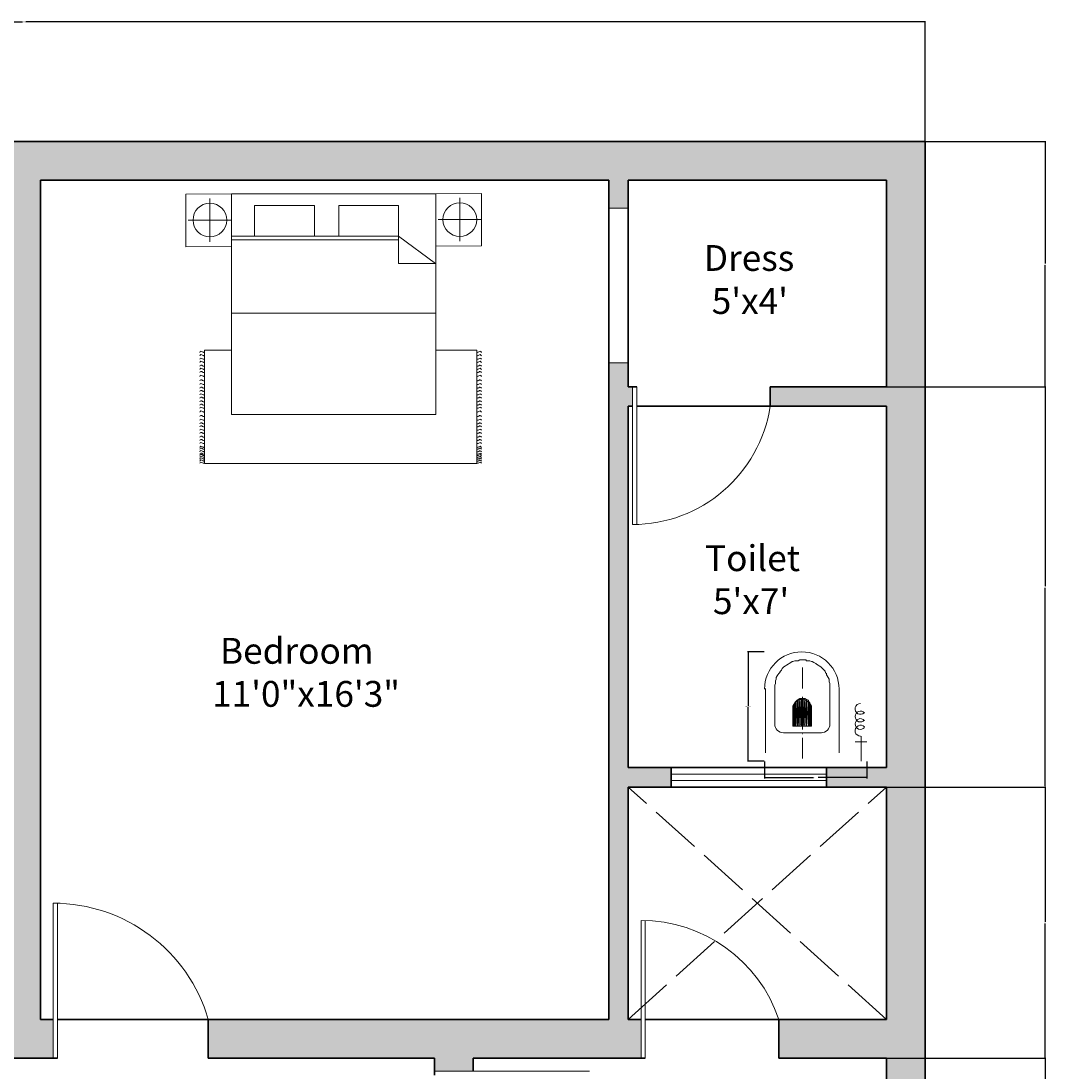
# Model space of a CAD drawing. Units: inches. Extents: x 1752 to 2227, y 6273 to 6884.
# Tile 6 of 6: x 1989 to 2227, y 6640 to 6884. Entities that reach past the tile are written whole.
import ezdxf

# ---------------------------------------------------------------- set-up
doc = ezdxf.new("R2010")
doc.units = ezdxf.units.IN
doc.header["$MEASUREMENT"] = 0
doc.linetypes.add('ACAD_ISO02W100', pattern=[15, 12, -3])
for name, color, linetype, lineweight in [('A-ANNO-DIMS', 2, 'Continuous', 18), ('A-AREA-IDEN', 7, 'Continuous', 18), ('A-DOOR', 3, 'Continuous', 20), ('A-FLOR-FIXT', 8, 'Continuous', 18), ('A-FLOR-VOID', 8, 'ACAD_ISO02W100', 13), ('A-FURN', 8, 'Continuous', 18), ('A-GLAZ', 4, 'Continuous', 18), ('A-WALL', 7, 'Continuous', 35), ('A-WALL-OPNG', 7, 'Continuous', 18)]:
    doc.layers.add(name, color=color, linetype=linetype, lineweight=lineweight)
doc.layers.add('A-WALL-PATT', color=32, linetype='Continuous', lineweight=13, true_color=0xcd6928)
doc.styles.get("Standard").update_dxf_attribs({"font": 'arial.ttf'})
doc.dimstyles.get("Standard").update_dxf_attribs({"dimtxt": 0.18, "dimasz": 0.18, "dimexe": 0.18, "dimexo": 0.0625, "dimgap": 0.09, "dimtad": 0, "dimtih": 1, "dimtoh": 1, "dimdec": 4, "dimzin": 0, "dimdsep": 46, "dimtxsty": 'Standard', "dimcen": 0.09, "dimadec": 0, "dimazin": 0, "dimtfac": 1, "dimtdec": 4, "dimtofl": 0, "dimtmove": 0, "dimatfit": 3, "dimfxl": 1, "dimtolj": 1, "dimtzin": 0, "dimarcsym": 0})

# ---------------------------------------------------------------- blocks, each defined once
blk = doc.blocks.new('BED-DOUBLE-SET')
for p, q in [((5.6, 61.62), (5.6, 51.56)), ((63.65, 61.72), (63.65, 51.66)), ((10.63, 56.59), (0.57, 56.59)), ((68.68, 56.69), (58.62, 56.69)), ((49.39, 52.82), (10.63, 52.82)), ((49.44, 52), (10.63, 52)), ((49.39, 52.82), (58, 46.47)), ((49.44, 52.82), (49.44, 46.47)), ((49.44, 46.47), (58, 46.47)), ((58.05, 34.96), (10.63, 34.96)), ((4.35, 0), (4.35, 26.37)), ((4.35, 26.37), (10.65, 26.37)), ((58.05, 26.37), (67.59, 26.37)), ((67.59, 26.37), (67.59, 0)), ((67.59, 0), (4.35, 0))]:
    blk.add_line(p, q)
for points in [[(0, 50.39), (10.63, 50.5), (10.63, 62.68), (0, 62.58)], [(58.05, 62.68), (58.05, 11.37), (10.63, 11.37), (10.63, 62.68)], [(58.05, 50.5), (68.68, 50.6), (68.68, 62.78), (58.05, 62.68)], [(29.88, 59.98), (29.88, 52.82), (15.98, 52.82), (15.98, 59.98)], [(49.44, 59.98), (49.44, 52.82), (35.55, 52.82), (35.55, 59.98)]]:
    blk.add_lwpolyline(points, close=True)
for centre in [(5.6, 56.59), (63.65, 56.69)]:
    blk.add_circle(centre, 3.92)
for points, knots in [([(3.23, 25.84), (3.32, 25.96), (3.52, 26.2), (3.86, 25.96), (4.14, 25.78), (4.29, 25.89), (4.35, 25.94)], [0, 0, 0, 0, 0.400747, 0.791423, 1.067667, 1.29709, 1.29709, 1.29709, 1.29709]), ([(3.23, 25.06), (3.32, 25.18), (3.52, 25.42), (3.86, 25.18), (4.14, 25.01), (4.29, 25.11), (4.35, 25.16)], [0, 0, 0, 0, 0.400747, 0.791423, 1.067667, 1.29709, 1.29709, 1.29709, 1.29709]), ([(3.23, 24.24), (3.32, 24.36), (3.52, 24.6), (3.86, 24.36), (4.14, 24.19), (4.29, 24.3), (4.35, 24.34)], [0, 0, 0, 0, 0.400747, 0.791423, 1.067667, 1.29709, 1.29709, 1.29709, 1.29709]), ([(68.71, 25.84), (68.61, 25.96), (68.42, 26.2), (68.08, 25.96), (67.8, 25.78), (67.65, 25.89), (67.58, 25.94)], [0, 0, 0, 0, 0.400747, 0.791423, 1.067667, 1.29709, 1.29709, 1.29709, 1.29709]), ([(68.71, 25.06), (68.61, 25.18), (68.42, 25.42), (68.08, 25.18), (67.8, 25.01), (67.65, 25.11), (67.58, 25.16)], [0, 0, 0, 0, 0.400747, 0.791423, 1.067667, 1.29709, 1.29709, 1.29709, 1.29709]), ([(68.71, 24.24), (68.61, 24.36), (68.42, 24.6), (68.08, 24.36), (67.8, 24.19), (67.65, 24.3), (67.58, 24.34)], [0, 0, 0, 0, 0.400747, 0.791423, 1.067667, 1.29709, 1.29709, 1.29709, 1.29709]), ([(3.23, 23.51), (3.32, 23.63), (3.52, 23.87), (3.86, 23.63), (4.14, 23.46), (4.29, 23.57), (4.35, 23.62)], [0, 0, 0, 0, 0.400747, 0.791423, 1.067667, 1.29709, 1.29709, 1.29709, 1.29709]), ([(3.23, 22.63), (3.32, 22.75), (3.52, 22.99), (3.86, 22.75), (4.14, 22.58), (4.29, 22.69), (4.35, 22.73)], [0, 0, 0, 0, 0.400747, 0.791423, 1.067667, 1.29709, 1.29709, 1.29709, 1.29709]), ([(3.23, 21.88), (3.32, 22), (3.52, 22.24), (3.86, 22), (4.14, 21.83), (4.29, 21.93), (4.35, 21.98)], [0, 0, 0, 0, 0.400747, 0.791423, 1.067667, 1.29709, 1.29709, 1.29709, 1.29709]), ([(68.71, 23.51), (68.61, 23.63), (68.42, 23.87), (68.08, 23.63), (67.8, 23.46), (67.65, 23.57), (67.58, 23.62)], [0, 0, 0, 0, 0.400747, 0.791423, 1.067667, 1.29709, 1.29709, 1.29709, 1.29709]), ([(68.71, 22.63), (68.61, 22.75), (68.42, 22.99), (68.08, 22.75), (67.8, 22.58), (67.65, 22.69), (67.58, 22.73)], [0, 0, 0, 0, 0.400747, 0.791423, 1.067667, 1.29709, 1.29709, 1.29709, 1.29709]), ([(68.71, 21.88), (68.61, 22), (68.42, 22.24), (68.08, 22), (67.8, 21.83), (67.65, 21.93), (67.58, 21.98)], [0, 0, 0, 0, 0.400747, 0.791423, 1.067667, 1.29709, 1.29709, 1.29709, 1.29709]), ([(3.23, 21.15), (3.32, 21.27), (3.52, 21.51), (3.86, 21.27), (4.14, 21.1), (4.29, 21.21), (4.35, 21.25)], [0, 0, 0, 0, 0.400747, 0.791423, 1.067667, 1.29709, 1.29709, 1.29709, 1.29709]), ([(3.23, 20.27), (3.32, 20.39), (3.52, 20.63), (3.86, 20.39), (4.14, 20.22), (4.29, 20.32), (4.35, 20.37)], [0, 0, 0, 0, 0.400747, 0.791423, 1.067667, 1.29709, 1.29709, 1.29709, 1.29709]), ([(68.71, 21.15), (68.61, 21.27), (68.42, 21.51), (68.08, 21.27), (67.8, 21.1), (67.65, 21.21), (67.58, 21.25)], [0, 0, 0, 0, 0.400747, 0.791423, 1.067667, 1.29709, 1.29709, 1.29709, 1.29709]), ([(68.71, 20.27), (68.61, 20.39), (68.42, 20.63), (68.08, 20.39), (67.8, 20.22), (67.65, 20.32), (67.58, 20.37)], [0, 0, 0, 0, 0.400747, 0.791423, 1.067667, 1.29709, 1.29709, 1.29709, 1.29709]), ([(3.23, 19.23), (3.32, 19.35), (3.52, 19.59), (3.86, 19.35), (4.14, 19.18), (4.29, 19.29), (4.35, 19.33)], [0, 0, 0, 0, 0.400747, 0.791423, 1.067667, 1.29709, 1.29709, 1.29709, 1.29709]), ([(3.23, 18.35), (3.32, 18.47), (3.52, 18.71), (3.86, 18.47), (4.14, 18.3), (4.29, 18.4), (4.35, 18.45)], [0, 0, 0, 0, 0.400747, 0.791423, 1.067667, 1.29709, 1.29709, 1.29709, 1.29709]), ([(3.23, 17.53), (3.32, 17.65), (3.52, 17.89), (3.86, 17.65), (4.14, 17.48), (4.29, 17.59), (4.35, 17.64)], [0, 0, 0, 0, 0.400747, 0.791423, 1.067667, 1.29709, 1.29709, 1.29709, 1.29709]), ([(68.71, 19.23), (68.61, 19.35), (68.42, 19.59), (68.08, 19.35), (67.8, 19.18), (67.65, 19.29), (67.58, 19.33)], [0, 0, 0, 0, 0.400747, 0.791423, 1.067667, 1.29709, 1.29709, 1.29709, 1.29709]), ([(68.71, 18.35), (68.61, 18.47), (68.42, 18.71), (68.08, 18.47), (67.8, 18.3), (67.65, 18.4), (67.58, 18.45)], [0, 0, 0, 0, 0.400747, 0.791423, 1.067667, 1.29709, 1.29709, 1.29709, 1.29709]), ([(68.71, 17.53), (68.61, 17.65), (68.42, 17.89), (68.08, 17.65), (67.8, 17.48), (67.65, 17.59), (67.58, 17.64)], [0, 0, 0, 0, 0.400747, 0.791423, 1.067667, 1.29709, 1.29709, 1.29709, 1.29709]), ([(3.23, 16.76), (3.32, 16.88), (3.52, 17.12), (3.86, 16.88), (4.14, 16.71), (4.29, 16.81), (4.35, 16.86)], [0, 0, 0, 0, 0.400747, 0.791423, 1.067667, 1.29709, 1.29709, 1.29709, 1.29709]), ([(3.23, 15.94), (3.32, 16.06), (3.52, 16.3), (3.86, 16.06), (4.14, 15.89), (4.29, 16), (4.35, 16.04)], [0, 0, 0, 0, 0.400747, 0.791423, 1.067667, 1.29709, 1.29709, 1.29709, 1.29709]), ([(3.23, 15.21), (3.32, 15.33), (3.52, 15.57), (3.86, 15.33), (4.14, 15.16), (4.29, 15.27), (4.35, 15.32)], [0, 0, 0, 0, 0.400747, 0.791423, 1.067667, 1.29709, 1.29709, 1.29709, 1.29709]), ([(68.71, 16.76), (68.61, 16.88), (68.42, 17.12), (68.08, 16.88), (67.8, 16.71), (67.65, 16.81), (67.58, 16.86)], [0, 0, 0, 0, 0.400747, 0.791423, 1.067667, 1.29709, 1.29709, 1.29709, 1.29709]), ([(68.71, 15.94), (68.61, 16.06), (68.42, 16.3), (68.08, 16.06), (67.8, 15.89), (67.65, 16), (67.58, 16.04)], [0, 0, 0, 0, 0.400747, 0.791423, 1.067667, 1.29709, 1.29709, 1.29709, 1.29709]), ([(68.71, 15.21), (68.61, 15.33), (68.42, 15.57), (68.08, 15.33), (67.8, 15.16), (67.65, 15.27), (67.58, 15.32)], [0, 0, 0, 0, 0.400747, 0.791423, 1.067667, 1.29709, 1.29709, 1.29709, 1.29709]), ([(3.23, 14.33), (3.32, 14.45), (3.52, 14.69), (3.86, 14.45), (4.14, 14.28), (4.29, 14.39), (4.35, 14.43)], [0, 0, 0, 0, 0.400747, 0.791423, 1.067667, 1.29709, 1.29709, 1.29709, 1.29709]), ([(3.23, 13.58), (3.32, 13.7), (3.52, 13.94), (3.86, 13.7), (4.14, 13.53), (4.29, 13.63), (4.35, 13.68)], [0, 0, 0, 0, 0.400747, 0.791423, 1.067667, 1.29709, 1.29709, 1.29709, 1.29709]), ([(3.23, 12.85), (3.32, 12.97), (3.52, 13.21), (3.86, 12.97), (4.14, 12.8), (4.29, 12.9), (4.35, 12.95)], [0, 0, 0, 0, 0.400747, 0.791423, 1.067667, 1.29709, 1.29709, 1.29709, 1.29709]), ([(3.23, 11.97), (3.32, 12.09), (3.52, 12.33), (3.86, 12.09), (4.14, 11.92), (4.29, 12.02), (4.35, 12.07)], [0, 0, 0, 0, 0.400747, 0.791423, 1.067667, 1.29709, 1.29709, 1.29709, 1.29709]), ([(68.71, 14.33), (68.61, 14.45), (68.42, 14.69), (68.08, 14.45), (67.8, 14.28), (67.65, 14.39), (67.58, 14.43)], [0, 0, 0, 0, 0.400747, 0.791423, 1.067667, 1.29709, 1.29709, 1.29709, 1.29709]), ([(68.71, 13.58), (68.61, 13.7), (68.42, 13.94), (68.08, 13.7), (67.8, 13.53), (67.65, 13.63), (67.58, 13.68)], [0, 0, 0, 0, 0.400747, 0.791423, 1.067667, 1.29709, 1.29709, 1.29709, 1.29709]), ([(68.71, 12.85), (68.61, 12.97), (68.42, 13.21), (68.08, 12.97), (67.8, 12.8), (67.65, 12.9), (67.58, 12.95)], [0, 0, 0, 0, 0.400747, 0.791423, 1.067667, 1.29709, 1.29709, 1.29709, 1.29709]), ([(68.71, 11.97), (68.61, 12.09), (68.42, 12.33), (68.08, 12.09), (67.8, 11.92), (67.65, 12.02), (67.58, 12.07)], [0, 0, 0, 0, 0.400747, 0.791423, 1.067667, 1.29709, 1.29709, 1.29709, 1.29709]), ([(3.23, 10.93), (3.32, 11.05), (3.52, 11.29), (3.86, 11.05), (4.14, 10.88), (4.29, 10.99), (4.35, 11.03)], [0, 0, 0, 0, 0.400747, 0.791423, 1.067667, 1.29709, 1.29709, 1.29709, 1.29709]), ([(3.23, 10.05), (3.32, 10.17), (3.52, 10.41), (3.86, 10.17), (4.14, 10), (4.29, 10.1), (4.35, 10.15)], [0, 0, 0, 0, 0.400747, 0.791423, 1.067667, 1.29709, 1.29709, 1.29709, 1.29709]), ([(68.71, 10.93), (68.61, 11.05), (68.42, 11.29), (68.08, 11.05), (67.8, 10.88), (67.65, 10.99), (67.58, 11.03)], [0, 0, 0, 0, 0.400747, 0.791423, 1.067667, 1.29709, 1.29709, 1.29709, 1.29709]), ([(68.71, 10.05), (68.61, 10.17), (68.42, 10.41), (68.08, 10.17), (67.8, 10), (67.65, 10.1), (67.58, 10.15)], [0, 0, 0, 0, 0.400747, 0.791423, 1.067667, 1.29709, 1.29709, 1.29709, 1.29709]), ([(3.23, 9.23), (3.32, 9.35), (3.52, 9.59), (3.86, 9.35), (4.14, 9.18), (4.29, 9.29), (4.35, 9.34)], [0, 0, 0, 0, 0.400747, 0.791423, 1.067667, 1.29709, 1.29709, 1.29709, 1.29709]), ([(3.23, 8.54), (3.32, 8.66), (3.52, 8.9), (3.86, 8.66), (4.14, 8.49), (4.29, 8.6), (4.35, 8.65)], [0, 0, 0, 0, 0.400747, 0.791423, 1.067667, 1.29709, 1.29709, 1.29709, 1.29709]), ([(3.23, 7.73), (3.32, 7.85), (3.52, 8.09), (3.86, 7.85), (4.14, 7.68), (4.29, 7.78), (4.35, 7.83)], [0, 0, 0, 0, 0.400747, 0.791423, 1.067667, 1.29709, 1.29709, 1.29709, 1.29709]), ([(68.71, 9.23), (68.61, 9.35), (68.42, 9.59), (68.08, 9.35), (67.8, 9.18), (67.65, 9.29), (67.58, 9.34)], [0, 0, 0, 0, 0.400747, 0.791423, 1.067667, 1.29709, 1.29709, 1.29709, 1.29709]), ([(68.71, 8.54), (68.61, 8.66), (68.42, 8.9), (68.08, 8.66), (67.8, 8.49), (67.65, 8.6), (67.58, 8.65)], [0, 0, 0, 0, 0.400747, 0.791423, 1.067667, 1.29709, 1.29709, 1.29709, 1.29709]), ([(68.71, 7.73), (68.61, 7.85), (68.42, 8.09), (68.08, 7.85), (67.8, 7.68), (67.65, 7.78), (67.58, 7.83)], [0, 0, 0, 0, 0.400747, 0.791423, 1.067667, 1.29709, 1.29709, 1.29709, 1.29709]), ([(3.23, 7), (3.32, 7.12), (3.52, 7.36), (3.86, 7.12), (4.14, 6.95), (4.29, 7.05), (4.35, 7.1)], [0, 0, 0, 0, 0.400747, 0.791423, 1.067667, 1.29709, 1.29709, 1.29709, 1.29709]), ([(3.23, 6.12), (3.32, 6.24), (3.52, 6.48), (3.86, 6.24), (4.14, 6.07), (4.29, 6.17), (4.35, 6.22)], [0, 0, 0, 0, 0.400747, 0.791423, 1.067667, 1.29709, 1.29709, 1.29709, 1.29709]), ([(3.23, 5.37), (3.32, 5.49), (3.52, 5.73), (3.86, 5.49), (4.14, 5.31), (4.29, 5.42), (4.35, 5.47)], [0, 0, 0, 0, 0.400747, 0.791423, 1.067667, 1.29709, 1.29709, 1.29709, 1.29709]), ([(3.23, 4.64), (3.32, 4.76), (3.52, 5), (3.86, 4.76), (4.14, 4.59), (4.29, 4.69), (4.35, 4.74)], [0, 0, 0, 0, 0.400747, 0.791423, 1.067667, 1.29709, 1.29709, 1.29709, 1.29709]), ([(68.71, 7), (68.61, 7.12), (68.42, 7.36), (68.08, 7.12), (67.8, 6.95), (67.65, 7.05), (67.58, 7.1)], [0, 0, 0, 0, 0.400747, 0.791423, 1.067667, 1.29709, 1.29709, 1.29709, 1.29709]), ([(68.71, 6.12), (68.61, 6.24), (68.42, 6.48), (68.08, 6.24), (67.8, 6.07), (67.65, 6.17), (67.58, 6.22)], [0, 0, 0, 0, 0.400747, 0.791423, 1.067667, 1.29709, 1.29709, 1.29709, 1.29709]), ([(68.71, 5.37), (68.61, 5.49), (68.42, 5.73), (68.08, 5.49), (67.8, 5.31), (67.65, 5.42), (67.58, 5.47)], [0, 0, 0, 0, 0.400747, 0.791423, 1.067667, 1.29709, 1.29709, 1.29709, 1.29709]), ([(68.71, 4.64), (68.61, 4.76), (68.42, 5), (68.08, 4.76), (67.8, 4.59), (67.66, 4.69), (67.59, 4.73)], [0, 0, 0, 0, 0.400747, 0.791423, 1.067667, 1.283686, 1.283686, 1.283686, 1.283686]), ([(3.23, 3.75), (3.32, 3.88), (3.52, 4.12), (3.86, 3.88), (4.14, 3.7), (4.29, 3.81), (4.35, 3.86)], [0, 0, 0, 0, 0.400747, 0.791423, 1.067667, 1.29709, 1.29709, 1.29709, 1.29709]), ([(3.23, 3.33), (3.32, 3.45), (3.52, 3.7), (3.86, 3.45), (4.14, 3.27), (4.29, 3.38), (4.35, 3.43)], [0, 0, 0, 0, 0.407265, 0.802015, 1.07826, 1.307683, 1.307683, 1.307683, 1.307683]), ([(3.23, 2.76), (3.32, 2.88), (3.52, 3.12), (3.86, 2.88), (4.14, 2.71), (4.29, 2.81), (4.35, 2.86)], [0, 0, 0, 0, 0.400747, 0.791423, 1.067667, 1.29709, 1.29709, 1.29709, 1.29709]), ([(3.23, 2.19), (3.32, 2.31), (3.52, 2.55), (3.86, 2.31), (4.14, 2.13), (4.29, 2.24), (4.35, 2.29)], [0, 0, 0, 0, 0.400747, 0.791423, 1.067667, 1.29709, 1.29709, 1.29709, 1.29709]), ([(68.71, 3.75), (68.61, 3.88), (68.42, 4.12), (68.08, 3.88), (67.8, 3.7), (67.66, 3.81), (67.59, 3.85)], [0, 0, 0, 0, 0.400747, 0.791423, 1.067667, 1.283686, 1.283686, 1.283686, 1.283686]), ([(68.71, 3.33), (68.61, 3.45), (68.42, 3.69), (68.08, 3.45), (67.8, 3.28), (67.66, 3.38), (67.59, 3.42)], [0, 0, 0, 0, 0.402903, 0.794912, 1.071156, 1.287177, 1.287177, 1.287177, 1.287177]), ([(68.71, 2.73), (68.61, 2.85), (68.42, 3.09), (68.08, 2.85), (67.8, 2.68), (67.66, 2.78), (67.59, 2.83)], [0, 0, 0, 0, 0.400747, 0.791423, 1.067667, 1.283686, 1.283686, 1.283686, 1.283686]), ([(3.23, 1.88), (3.32, 2), (3.52, 2.24), (3.86, 2), (4.14, 1.82), (4.29, 1.93), (4.35, 1.98)], [0, 0, 0, 0, 0.400747, 0.791423, 1.067667, 1.29709, 1.29709, 1.29709, 1.29709]), ([(3.23, 1.46), (3.32, 1.58), (3.52, 1.82), (3.86, 1.58), (4.14, 1.41), (4.29, 1.51), (4.35, 1.56)], [0, 0, 0, 0, 0.400747, 0.791423, 1.067667, 1.29709, 1.29709, 1.29709, 1.29709]), ([(3.23, 1.06), (3.32, 1.18), (3.52, 1.42), (3.86, 1.18), (4.14, 1.01), (4.29, 1.11), (4.35, 1.16)], [0, 0, 0, 0, 0.400747, 0.791423, 1.067667, 1.29709, 1.29709, 1.29709, 1.29709]), ([(3.23, 0.57), (3.32, 0.7), (3.52, 0.94), (3.86, 0.7), (4.14, 0.52), (4.29, 0.63), (4.35, 0.68)], [0, 0, 0, 0, 0.400747, 0.791423, 1.067667, 1.29709, 1.29709, 1.29709, 1.29709]), ([(3.23, 0.07), (3.32, 0.19), (3.52, 0.43), (3.86, 0.19), (4.14, 0.02), (4.29, 0.13), (4.35, 0.18)], [0, 0, 0, 0, 0.400747, 0.791423, 1.067667, 1.29709, 1.29709, 1.29709, 1.29709]), ([(68.71, 1.43), (68.61, 1.55), (68.42, 1.79), (68.08, 1.55), (67.8, 1.38), (67.65, 1.48), (67.58, 1.53)], [0, 0, 0, 0, 0.400747, 0.791423, 1.067667, 1.29709, 1.29709, 1.29709, 1.29709]), ([(68.71, 1.03), (68.61, 1.15), (68.42, 1.39), (68.08, 1.15), (67.8, 0.98), (67.65, 1.09), (67.58, 1.13)], [0, 0, 0, 0, 0.400747, 0.791423, 1.067667, 1.29709, 1.29709, 1.29709, 1.29709]), ([(68.71, 0.55), (68.61, 0.67), (68.42, 0.91), (68.08, 0.67), (67.8, 0.5), (67.65, 0.6), (67.58, 0.65)], [0, 0, 0, 0, 0.400747, 0.791423, 1.067667, 1.29709, 1.29709, 1.29709, 1.29709]), ([(68.71, 0.07), (68.61, 0.19), (68.42, 0.43), (68.08, 0.19), (67.8, 0.02), (67.65, 0.13), (67.58, 0.18)], [0, 0, 0, 0, 0.400747, 0.791423, 1.067667, 1.29709, 1.29709, 1.29709, 1.29709]), ([(68.71, 2.16), (68.61, 2.28), (68.42, 2.52), (68.08, 2.28), (67.8, 2.11), (67.66, 2.21), (67.59, 2.25)], [0, 0, 0, 0, 0.400747, 0.791423, 1.067667, 1.283686, 1.283686, 1.283686, 1.283686]), ([(68.71, 1.85), (68.61, 1.97), (68.42, 2.21), (68.08, 1.97), (67.8, 1.8), (67.66, 1.9), (67.59, 1.94)], [0, 0, 0, 0, 0.400747, 0.791423, 1.067667, 1.283686, 1.283686, 1.283686, 1.283686])]:
    blk.add_open_spline(points, degree=3, knots=knots)
blk = doc.blocks.new('WC-PLAN')
h = blk.add_hatch(color=256)
h.paths.add_polyline_path([(8.12, 16.94), (13.2, 16.94), (8.12, 17.17)])
h.paths.add_polyline_path([(13.2, 16.94), (8.12, 17.17), (12.82, 17.17)])
h.paths.add_polyline_path([(8.12, 17.17), (12.82, 17.17), (12.44, 17.17)])
h = blk.add_hatch(color=256)
h.paths.add_polyline_path([(8.12, 16.71), (13.58, 16.71), (8.12, 16.94)])
h.paths.add_polyline_path([(13.58, 16.71), (8.12, 16.94), (13.2, 16.94)])
h = blk.add_hatch(color=256)
h.paths.add_polyline_path([(8.12, 16.56), (13.81, 16.56), (8.12, 16.71)])
h.paths.add_polyline_path([(13.81, 16.56), (8.12, 16.71), (13.58, 16.71)])
h = blk.add_hatch(color=256)
h.paths.add_polyline_path([(8.12, 16.18), (14.19, 16.18), (8.12, 16.56)])
h.paths.add_polyline_path([(14.19, 16.18), (8.12, 16.56), (13.81, 16.56)])
h = blk.add_hatch(color=256)
h.paths.add_polyline_path([(8.12, 15.95), (14.34, 15.95), (8.12, 16.18)])
h.paths.add_polyline_path([(14.34, 15.95), (8.12, 16.18), (14.19, 16.18)])
h = blk.add_hatch(color=256)
h.paths.add_polyline_path([(8.12, 15.57), (14.56, 15.57), (8.12, 15.95)])
h.paths.add_polyline_path([(14.56, 15.57), (8.12, 15.95), (14.34, 15.95)])
h = blk.add_hatch(color=256)
h.paths.add_polyline_path([(8.12, 15.19), (14.56, 15.19), (8.12, 15.57)])
h.paths.add_polyline_path([(14.56, 15.19), (8.12, 15.57), (14.56, 15.57)])
h = blk.add_hatch(color=256)
h.paths.add_polyline_path([(8.12, 14.81), (14.56, 14.81), (8.12, 15.19)])
h.paths.add_polyline_path([(14.56, 14.81), (8.12, 15.19), (14.56, 15.19)])
h = blk.add_hatch(color=256)
h.paths.add_polyline_path([(8.12, 14.44), (14.56, 14.44), (8.12, 14.81)])
h.paths.add_polyline_path([(14.56, 14.44), (8.12, 14.81), (14.56, 14.81)])
h = blk.add_hatch(color=256)
h.paths.add_polyline_path([(8.12, 14.06), (14.34, 14.06), (8.12, 14.44)])
h.paths.add_polyline_path([(14.34, 14.06), (8.12, 14.44), (14.56, 14.44)])
h = blk.add_hatch(color=256)
h.paths.add_polyline_path([(8.12, 13.6), (14.19, 13.6), (8.12, 14.06)])
h.paths.add_polyline_path([(14.19, 13.6), (8.12, 14.06), (14.34, 14.06)])
h = blk.add_hatch(color=256)
h.paths.add_polyline_path([(8.12, 13.45), (13.81, 13.45), (8.12, 13.6)])
h.paths.add_polyline_path([(13.81, 13.45), (8.12, 13.6), (14.19, 13.6)])
h = blk.add_hatch(color=256)
h.paths.add_polyline_path([(8.12, 13.22), (13.58, 13.22), (8.12, 13.45)])
h.paths.add_polyline_path([(13.58, 13.22), (8.12, 13.45), (13.81, 13.45)])
h = blk.add_hatch(color=256)
h.paths.add_polyline_path([(8.12, 13.07), (13.2, 13.07), (8.12, 13.22)])
h.paths.add_polyline_path([(13.2, 13.07), (8.12, 13.22), (13.58, 13.22)])
h = blk.add_hatch(color=256)
h.paths.add_polyline_path([(8.12, 12.84), (12.82, 12.84), (8.12, 13.07)])
h.paths.add_polyline_path([(12.82, 12.84), (8.12, 13.07), (13.2, 13.07)])
for points in [[(1.9, 23.54), (16.92, 23.54), (16.92, 23.54)], [(8.72, 21.41), (15.93, 21.41), (15.93, 21.41)], [(15.93, 21.41), (16.69, 21.41), (17.3, 21.41), (17.67, 21.41), (18.05, 21.19), (18.43, 21.19), (18.66, 21.19), (19.04, 21.04), (19.42, 21.04), (19.8, 20.81), (20.03, 20.66), (20.41, 20.43), (20.56, 20.28), (20.94, 20.05), (21.16, 19.82), (21.54, 19.67), (21.77, 19.44), (21.92, 19.29), (22.15, 18.91), (22.3, 18.68), (22.53, 18.3), (22.68, 18.08), (22.91, 17.7), (23.14, 17.32), (23.14, 17.17), (23.29, 16.71), (23.29, 16.33), (23.29, 15.95), (23.52, 15.57), (23.52, 14.97), (23.52, 14.21), (23.29, 14.06), (23.29, 13.6), (23.29, 13.22), (23.14, 12.84), (23.14, 12.69), (22.91, 12.31), (22.68, 11.86), (22.53, 11.7), (22.3, 11.33), (22.15, 11.1), (21.92, 10.72), (21.77, 10.57), (21.54, 10.34), (21.16, 9.96), (20.94, 9.73), (20.56, 9.58), (20.41, 9.35), (20.03, 9.35), (19.8, 9.2), (19.42, 8.97), (19.04, 8.75), (18.66, 8.75), (18.43, 8.75), (18.05, 8.59), (17.67, 8.59), (17.3, 8.59), (16.69, 8.59), (15.93, 8.59)], [(6.6, 19.29), (6.6, 10.57), (6.6, 10.57)], [(8.12, 17.17), (8.12, 12.84), (8.12, 12.84)], [(8.12, 17.17), (12.44, 17.17), (12.44, 17.17)], [(0.61, 14.97), (5.46, 14.97), (5.46, 14.97)], [(6.37, 14.97), (6.37, 15.04), (6.37, 15.04)], [(7.36, 14.97), (14.94, 14.97), (14.94, 14.97)], [(8.57, 15.42), (8.5, 15.42), (8.5, 15.42)], [(8.57, 14.97), (8.5, 15.04), (8.5, 15.04)], [(8.57, 15.42), (8.57, 15.19), (8.57, 14.97)], [(8.57, 14.97), (8.57, 14.81), (8.57, 14.59)], [(16.92, 14.97), (21.77, 14.97), (21.77, 14.97)], [(8.12, 12.84), (12.44, 12.84), (12.44, 12.84)], [(8.57, 14.59), (8.5, 14.59), (8.5, 14.59)], [(8.72, 8.59), (15.93, 8.59), (15.93, 8.59)], [(1.9, 6.47), (16.92, 6.47), (16.92, 6.47)], [(4.48, 2.73), (4.48, 0), (4.48, 0)], [(0, 1.37), (5.84, 1.37), (5.84, 1.37)]]:
    blk.add_lwpolyline(points)
for points in [[(8.12, 16.94), (13.2, 16.94), (8.12, 17.17)], [(13.2, 16.94), (8.12, 17.17), (12.82, 17.17)], [(8.12, 17.17), (12.82, 17.17), (12.44, 17.17)], [(12.82, 17.17), (8.12, 17.17), (8.12, 17.17)], [(8.12, 16.71), (13.58, 16.71), (8.12, 16.94)], [(13.58, 16.71), (8.12, 16.94), (13.2, 16.94)], [(8.12, 16.56), (13.81, 16.56), (8.12, 16.71)], [(13.81, 16.56), (8.12, 16.71), (13.58, 16.71)], [(8.12, 16.18), (14.19, 16.18), (8.12, 16.56)], [(14.19, 16.18), (8.12, 16.56), (13.81, 16.56)], [(8.12, 15.95), (14.34, 15.95), (8.12, 16.18)], [(14.34, 15.95), (8.12, 16.18), (14.19, 16.18)], [(8.12, 15.57), (14.56, 15.57), (8.12, 15.95)], [(14.56, 15.57), (8.12, 15.95), (14.34, 15.95)], [(8.12, 15.19), (14.56, 15.19), (8.12, 15.57)], [(14.56, 15.19), (8.12, 15.57), (14.56, 15.57)], [(8.12, 14.81), (14.56, 14.81), (8.12, 15.19)], [(14.56, 14.81), (8.12, 15.19), (14.56, 15.19)], [(8.12, 14.44), (14.56, 14.44), (8.12, 14.81)], [(14.56, 14.44), (8.12, 14.81), (14.56, 14.81)], [(8.12, 14.06), (14.34, 14.06), (8.12, 14.44)], [(14.34, 14.06), (8.12, 14.44), (14.56, 14.44)], [(8.12, 13.6), (14.19, 13.6), (8.12, 14.06)], [(14.19, 13.6), (8.12, 14.06), (14.34, 14.06)], [(8.12, 13.45), (13.81, 13.45), (8.12, 13.6)], [(13.81, 13.45), (8.12, 13.6), (14.19, 13.6)], [(8.12, 13.22), (13.58, 13.22), (8.12, 13.45)], [(13.58, 13.22), (8.12, 13.45), (13.81, 13.45)], [(8.12, 13.07), (13.2, 13.07), (8.12, 13.22)], [(13.2, 13.07), (8.12, 13.22), (13.58, 13.22)], [(8.12, 12.84), (12.82, 12.84), (8.12, 13.07)], [(12.82, 12.84), (8.12, 13.07), (13.2, 13.07)], [(8.12, 12.84), (12.44, 12.84)], [(12.44, 12.84), (8.12, 12.84), (12.82, 12.84)]]:
    blk.add_lwpolyline(points, close=True)
for points, knots in [([(16.76, 6.47), (21.54, 6.47), (25.41, 10.34), (25.41, 15.12), (25.41, 15.12), (25.41, 19.9), (21.54, 23.77), (16.76, 23.77)], [0, 0, 0, 0, 0.125, 0.125, 0.125, 0.125001, 1, 1, 1, 1]), ([(12.29, 13.07), (13.43, 13.07), (14.34, 13.98), (14.34, 15.12), (14.34, 15.12), (14.34, 16.26), (13.43, 17.17), (12.29, 17.17)], [0, 0, 0, 0, 0.125, 0.125, 0.125, 0.125001, 1, 1, 1, 1]), ([(7.97, 0.53), (8.34, 0.91), (8.5, 1.59), (8.19, 2.05), (8.19, 2.05), (7.89, 2.58), (7.36, 2.88), (6.75, 2.73), (6.75, 2.73), (6.22, 2.58), (5.84, 2.05), (5.84, 1.52)], [0, 0, 0, 0, 0.083333, 0.083333, 0.083333, 0.083334, 0.166667, 0.166667, 0.166667, 0.166668, 1, 1, 1, 1]), ([(9.48, 0.61), (9.86, 0.91), (10.01, 1.52), (9.79, 1.97), (9.79, 1.97), (9.63, 2.43), (9.1, 2.73), (8.65, 2.73), (8.65, 2.73), (8.12, 2.73), (7.66, 2.43), (7.43, 1.97), (7.43, 1.97), (7.28, 1.44), (7.43, 0.91), (7.81, 0.53)], [0, 0, 0, 0, 0.0625, 0.0625, 0.0625, 0.062501, 0.125, 0.125, 0.125, 0.125001, 0.1875, 0.1875, 0.1875, 0.187501, 1, 1, 1, 1]), ([(11.23, 0.53), (11.61, 0.91), (11.76, 1.44), (11.53, 1.97), (11.53, 1.97), (11.38, 2.43), (10.92, 2.73), (10.39, 2.73), (10.39, 2.73), (9.86, 2.73), (9.41, 2.43), (9.18, 1.97), (9.18, 1.97), (9.03, 1.44), (9.18, 0.91), (9.56, 0.53)], [0, 0, 0, 0, 0.0625, 0.0625, 0.0625, 0.062501, 0.125, 0.125, 0.125, 0.125001, 0.1875, 0.1875, 0.1875, 0.187501, 1, 1, 1, 1]), ([(13.43, 1.52), (13.43, 2.05), (12.97, 2.58), (12.44, 2.73), (12.44, 2.73), (11.91, 2.88), (11.3, 2.58), (11, 2.12), (11, 2.12), (10.77, 1.59), (10.85, 0.99), (11.23, 0.61)], [0, 0, 0, 0, 0.083333, 0.083333, 0.083333, 0.083334, 0.166667, 0.166667, 0.166667, 0.166668, 1, 1, 1, 1])]:
    blk.add_open_spline(points, degree=3, knots=knots)
for points in [[(8.65, 21.41), (7.51, 21.41), (6.6, 20.5), (6.6, 19.37)], [(6.6, 10.64), (6.6, 9.5), (7.51, 8.59), (8.65, 8.59)]]:
    blk.add_open_spline(points, degree=3)
blk = doc.blocks.new('DOOR-SINGLE-36IN')
for p, q in [((35, 36), (35, 0)), ((36, 0), (36, 36)), ((36, 0), (35, 0))]:
    blk.add_line(p, q)
blk.add_arc((36, -1.5), 37.5, 90, 163.7398)
blk = doc.blocks.new('DOOR-SINGLE-32IN')
for p, q in [((32, 32), (31, 32)), ((31, 0), (31, 32)), ((32, 32), (32, 0))]:
    blk.add_line(p, q)
blk.add_arc((32, 33.76), 33.76, 198.5866, 270)
blk = doc.blocks.new('*D26')
at = {"layer": 'A-ANNO-DIMS', "color": 0, "lineweight": -2, "transparency": 16777216}
for p, q in [((2161.28, 6737.33), (2157.35, 6737.33)), ((2157.53, 6737.15), (2157.53, 6724.81)), ((2157.53, 6712.1), (2157.53, 6724.44)), ((2161.28, 6711.92), (2157.35, 6711.92))]:
    blk.add_line(p, q, dxfattribs=at)
at = {"layer": 'A-ANNO-DIMS', "color": 0, "transparency": 16777216}
for points in [[(2157.5, 6737.15), (2157.56, 6737.15), (2157.53, 6737.33)], [(2157.5, 6712.1), (2157.56, 6712.1), (2157.53, 6711.92)]]:
    blk.add_solid(points, dxfattribs=at)
at = {"layer": 'Defpoints', "color": 0, "transparency": 16777216}
for p in [(2157.53, 6737.33), (2161.34, 6737.33), (2161.34, 6711.92)]:
    blk.add_point(p, dxfattribs=at)
at = {"layer": 'A-ANNO-DIMS', "color": 0, "transparency": 16777216, "insert": (2157.53, 6724.63), "char_height": 0.18, "attachment_point": 5}
blk.add_mtext('\\A1;WC 25 TYP.', dxfattribs=at)
blk = doc.blocks.new('*D27')
at = {"layer": 'A-ANNO-DIMS', "color": 0, "lineweight": -2, "transparency": 16777216}
for p, q in [((2161.34, 6711.86), (2161.34, 6707.93)), ((2185.11, 6711.86), (2185.11, 6707.93)), ((2161.52, 6708.11), (2172.7, 6708.11)), ((2184.93, 6708.11), (2173.76, 6708.11))]:
    blk.add_line(p, q, dxfattribs=at)
at = {"layer": 'A-ANNO-DIMS', "color": 0, "transparency": 16777216}
for points in [[(2161.52, 6708.14), (2161.52, 6708.08), (2161.34, 6708.11)], [(2184.93, 6708.14), (2184.93, 6708.08), (2185.11, 6708.11)]]:
    blk.add_solid(points, dxfattribs=at)
at = {"layer": 'Defpoints', "color": 0, "transparency": 16777216}
for p in [(2161.34, 6711.92), (2185.11, 6711.92), (2161.34, 6708.11)]:
    blk.add_point(p, dxfattribs=at)
at = {"layer": 'A-ANNO-DIMS', "color": 0, "transparency": 16777216, "insert": (2173.23, 6708.11), "char_height": 0.18, "attachment_point": 5}
blk.add_mtext('\\A1;24 TYP.', dxfattribs=at)
blk = doc.blocks.new('*D40')
at = {"layer": 'A-ANNO-DIMS', "color": 0, "lineweight": -2, "transparency": 16777216}
for p, q in [((1780.15, 6855.98), (1780.15, 6883.94)), ((1780.33, 6883.76), (1989, 6883.76)), ((2198.47, 6883.76), (1989.8, 6883.76)), ((2198.65, 6855.98), (2198.65, 6883.94))]:
    blk.add_line(p, q, dxfattribs=at)
at = {"layer": 'A-ANNO-DIMS', "color": 0, "transparency": 16777216}
for points in [[(1780.33, 6883.79), (1780.33, 6883.73), (1780.15, 6883.76)], [(2198.47, 6883.79), (2198.47, 6883.73), (2198.65, 6883.76)]]:
    blk.add_solid(points, dxfattribs=at)
at = {"layer": 'Defpoints', "color": 0, "transparency": 16777216}
for p in [(2198.65, 6883.76), (1780.15, 6855.91), (2198.65, 6855.91)]:
    blk.add_point(p, dxfattribs=at)
at = {"layer": 'A-ANNO-DIMS', "color": 0, "transparency": 16777216, "insert": (1989.4, 6883.76), "char_height": 0.18, "attachment_point": 5}
blk.add_mtext('\\A1;418.5', dxfattribs=at)
blk = doc.blocks.new('*D43')
at = {"layer": 'A-ANNO-DIMS', "color": 0, "lineweight": -2, "transparency": 16777216}
for p, q in [((2189.71, 6642.91), (2226.68, 6642.91)), ((2226.5, 6642.73), (2226.5, 6572.59)), ((2226.5, 6502.09), (2226.5, 6572.23)), ((2189.71, 6501.91), (2226.68, 6501.91))]:
    blk.add_line(p, q, dxfattribs=at)
at = {"layer": 'A-ANNO-DIMS', "color": 0, "transparency": 16777216}
for points in [[(2226.47, 6642.73), (2226.53, 6642.73), (2226.5, 6642.91)], [(2226.47, 6502.09), (2226.53, 6502.09), (2226.5, 6501.91)]]:
    blk.add_solid(points, dxfattribs=at)
at = {"layer": 'Defpoints', "color": 0, "transparency": 16777216}
for p in [(2189.65, 6642.91), (2226.5, 6642.91), (2189.65, 6501.91)]:
    blk.add_point(p, dxfattribs=at)
at = {"layer": 'A-ANNO-DIMS', "color": 0, "transparency": 16777216, "insert": (2226.5, 6572.41), "char_height": 0.18, "attachment_point": 5}
blk.add_mtext('\\A1;141', dxfattribs=at)
blk = doc.blocks.new('*D44')
at = {"layer": 'A-ANNO-DIMS', "color": 0, "lineweight": -2, "transparency": 16777216}
for p, q in [((2189.71, 6705.91), (2226.68, 6705.91)), ((2226.5, 6705.73), (2226.5, 6674.6)), ((2226.5, 6643.09), (2226.5, 6674.23)), ((2189.71, 6642.91), (2226.68, 6642.91))]:
    blk.add_line(p, q, dxfattribs=at)
at = {"layer": 'A-ANNO-DIMS', "color": 0, "transparency": 16777216}
for points in [[(2226.47, 6705.73), (2226.53, 6705.73), (2226.5, 6705.91)], [(2226.47, 6643.09), (2226.53, 6643.09), (2226.5, 6642.91)]]:
    blk.add_solid(points, dxfattribs=at)
at = {"layer": 'Defpoints', "color": 0, "transparency": 16777216}
for p in [(2189.65, 6705.91), (2226.5, 6705.91), (2189.65, 6642.91)]:
    blk.add_point(p, dxfattribs=at)
at = {"layer": 'A-ANNO-DIMS', "color": 0, "transparency": 16777216, "insert": (2226.5, 6674.41), "char_height": 0.18, "attachment_point": 5}
blk.add_mtext('\\A1;63', dxfattribs=at)
blk = doc.blocks.new('*D45')
at = {"layer": 'A-ANNO-DIMS', "color": 0, "lineweight": -2, "transparency": 16777216}
for p, q in [((2189.71, 6798.91), (2226.68, 6798.91)), ((2226.5, 6798.73), (2226.5, 6752.6)), ((2226.5, 6706.09), (2226.5, 6752.23)), ((2189.71, 6705.91), (2226.68, 6705.91))]:
    blk.add_line(p, q, dxfattribs=at)
at = {"layer": 'A-ANNO-DIMS', "color": 0, "transparency": 16777216}
for points in [[(2226.47, 6798.73), (2226.53, 6798.73), (2226.5, 6798.91)], [(2226.47, 6706.09), (2226.53, 6706.09), (2226.5, 6705.91)]]:
    blk.add_solid(points, dxfattribs=at)
at = {"layer": 'Defpoints', "color": 0, "transparency": 16777216}
for p in [(2189.65, 6798.91), (2226.5, 6798.91), (2189.65, 6705.91)]:
    blk.add_point(p, dxfattribs=at)
at = {"layer": 'A-ANNO-DIMS', "color": 0, "transparency": 16777216, "insert": (2226.5, 6752.41), "char_height": 0.18, "attachment_point": 5}
blk.add_mtext('\\A1;93', dxfattribs=at)
blk = doc.blocks.new('*D46')
at = {"layer": 'A-ANNO-DIMS', "color": 0, "lineweight": -2, "transparency": 16777216}
for p, q in [((2198.71, 6855.91), (2226.68, 6855.91)), ((2226.5, 6855.73), (2226.5, 6827.6)), ((2226.5, 6799.09), (2226.5, 6827.23)), ((2189.71, 6798.91), (2226.68, 6798.91))]:
    blk.add_line(p, q, dxfattribs=at)
at = {"layer": 'A-ANNO-DIMS', "color": 0, "transparency": 16777216}
for points in [[(2226.47, 6855.73), (2226.53, 6855.73), (2226.5, 6855.91)], [(2226.47, 6799.09), (2226.53, 6799.09), (2226.5, 6798.91)]]:
    blk.add_solid(points, dxfattribs=at)
at = {"layer": 'Defpoints', "color": 0, "transparency": 16777216}
for p in [(2198.65, 6855.91), (2226.5, 6855.91), (2189.65, 6798.91)]:
    blk.add_point(p, dxfattribs=at)
at = {"layer": 'A-ANNO-DIMS', "color": 0, "transparency": 16777216, "insert": (2226.5, 6827.41), "char_height": 0.18, "attachment_point": 5}
blk.add_mtext('\\A1;57', dxfattribs=at)

msp = doc.modelspace()

# ---------------------------------------------------------------- hatches: boundary and pattern name
at = {"layer": 'A-WALL-PATT'}
h = msp.add_hatch(color=256, dxfattribs=at)
h.dxf.hatch_style = 1
h.paths.add_polyline_path([(2198.6473, 6855.914), (1780.1473, 6855.914), (1780.1473, 6309.914), (1824.3861, 6309.914), (1824.3861, 6318.914), (1789.1473, 6318.914), (1789.1473, 6501.914), (1790.1473, 6501.914), (1790.1473, 6510.914), (1789.1473, 6510.914), (1789.1473, 6570.914), (1838.6473, 6570.914), (1838.6473, 6510.914), (1822.1473, 6510.914), (1822.1473, 6501.914), (1921.1473, 6501.914), (1921.1473, 6498.914), (1930.1473, 6498.914), (1930.1473, 6501.914), (1930.1473, 6510.914), (1847.6473, 6510.914), (1847.6473, 6585.039), (1838.6473, 6585.039), (1838.6473, 6575.414), (1789.1473, 6575.414), (1789.1473, 6705.914), (1795.2039, 6705.914), (1795.2039, 6714.914), (1789.1473, 6714.914), (1789.1473, 6846.914), (1984.1473, 6846.914), (1984.1473, 6714.914), (1977.8419, 6714.914), (1977.8419, 6705.914), (1984.1473, 6705.914), (1984.1473, 6651.914), (1977.6147, 6651.914), (1977.6147, 6642.914), (1996.1473, 6642.914), (1996.1473, 6651.914), (1993.1473, 6651.914), (1993.1473, 6846.914), (2125.1473, 6846.914), (2125.1473, 6840.4779), (2129.6473, 6840.4779), (2129.6473, 6846.914), (2189.6473, 6846.914), (2189.6473, 6798.914), (2162.6473, 6798.914), (2162.6473, 6794.414), (2189.6473, 6794.414), (2189.6473, 6710.414), (2175.6868, 6710.414), (2175.6868, 6705.914), (2189.6473, 6705.914), (2189.6473, 6651.914), (2164.6473, 6651.914), (2164.6473, 6642.914), (2189.6473, 6642.914), (2189.6473, 6510.914), (2166.7624, 6510.914), (2166.7624, 6501.914), (2189.6473, 6501.914), (2189.6473, 6318.914), (2173.9269, 6318.914), (2173.9269, 6309.914), (2198.6473, 6309.914)])
h.paths.add_polyline_path([(2023.6785, 6318.914), (1930.1473, 6318.914), (1930.1473, 6321.914), (1921.1473, 6321.914), (1921.1473, 6318.914), (1872.3861, 6318.914), (1872.3861, 6309.914), (2023.6785, 6309.914)], flags=17)
h.paths.add_polyline_path([(2092.7496, 6318.914), (2061.7431, 6318.914), (2061.7431, 6309.914), (2092.7496, 6309.914)], flags=0)
h.paths.add_polyline_path([(1947.0033, 6375.914), (1930.1473, 6375.914), (1930.1473, 6462.914), (1921.1473, 6462.914), (1921.1473, 6357.914), (1930.1473, 6357.914), (1930.1473, 6366.914), (1947.0033, 6366.914)], flags=17)
h.paths.add_polyline_path([(2024.6473, 6432.914), (2015.6473, 6432.914), (2015.6473, 6375.914), (1995.0033, 6375.914), (1995.0033, 6366.914), (2024.6473, 6366.914)], flags=17)
h.paths.add_polyline_path([(2030.6473, 6441.914), (2024.6473, 6441.914), (2024.6473, 6510.914), (2015.6473, 6510.914), (2015.6473, 6432.914), (2024.6473, 6432.914), (2030.6473, 6432.914)], flags=17)
h.paths.add_polyline_path([(2093.6473, 6501.914), (2118.7624, 6501.914), (2118.7624, 6510.914), (2093.6473, 6510.914), (2093.6473, 6603.914), (2084.6473, 6603.914), (2084.6473, 6441.914), (2078.6473, 6441.914), (2078.6473, 6432.914), (2093.6473, 6432.914)], flags=17)
h.paths.add_polyline_path([(2132.6473, 6651.914), (2129.6473, 6651.914), (2129.6473, 6705.914), (2139.6868, 6705.914), (2139.6868, 6710.414), (2129.6473, 6710.414), (2129.6473, 6794.414), (2130.6473, 6794.414), (2130.6473, 6798.914), (2129.6473, 6798.914), (2129.6473, 6804.4779), (2125.1473, 6804.4779), (2125.1473, 6651.914), (2032.1473, 6651.914), (2032.1473, 6642.914), (2084.6473, 6642.914), (2084.6473, 6639.914), (2093.6473, 6639.914), (2093.6473, 6642.914), (2132.6473, 6642.914)], flags=17)
h.paths.add_polyline_path([(1929.6147, 6651.914), (1924.1473, 6651.914), (1924.1473, 6705.914), (1941.8419, 6705.914), (1941.8419, 6714.914), (1911.8299, 6714.914), (1911.8299, 6705.914), (1919.6473, 6705.914), (1919.6473, 6651.914), (1847.6473, 6651.914), (1847.6473, 6662.4635), (1838.6473, 6662.4635), (1838.6473, 6621.039), (1847.6473, 6621.039), (1847.6473, 6642.914), (1929.6147, 6642.914)], flags=17)
h.paths.add_polyline_path([(1879.8299, 6714.914), (1831.2039, 6714.914), (1831.2039, 6705.914), (1838.6473, 6705.914), (1838.6473, 6698.4635), (1847.6473, 6698.4635), (1847.6473, 6705.914), (1879.8299, 6705.914)], flags=17)

# ---------------------------------------------------------------- linework, layer by layer
at = {"layer": 'A-DOOR'}
for p, q in [((2130.6473, 6798.914), (2130.6473, 6766.914)), ((2130.6473, 6766.914), (2130.6473, 6798.914)), ((2130.6473, 6798.914), (2131.6473, 6798.914)), ((2131.6473, 6766.914), (2131.6473, 6798.914)), ((1996.1473, 6678.914), (1996.1473, 6642.914)), ((2132.6473, 6674.914), (2132.6473, 6642.914)), ((2120.6473, 6639.914), (2084.6473, 6639.914))]:
    msp.add_line(p, q, dxfattribs=at)
msp.add_arc((2130.6473, 6799.2822), 32.3682, 270, 351.349879, dxfattribs=at)
at = {"layer": 'A-FLOR-VOID'}
for p, q in [((2129.6473, 6651.914), (2189.6473, 6705.914)), ((2189.6473, 6651.914), (2129.6473, 6705.914))]:
    msp.add_line(p, q, dxfattribs=at)
at = {"layer": 'A-GLAZ'}
for p, q in [((2175.6868, 6710.414), (2139.6868, 6710.414)), ((2175.6868, 6708.914), (2139.6868, 6708.914)), ((2139.6868, 6707.414), (2175.6868, 6707.414)), ((2139.6868, 6705.914), (2175.6868, 6705.914))]:
    msp.add_line(p, q, dxfattribs=at)
at = {"layer": 'A-WALL'}
for p, q in [((1780.1473, 6855.914), (2198.6473, 6855.914)), ((2198.6473, 6855.914), (2198.6473, 6309.914)), ((1993.1473, 6846.914), (1993.1473, 6651.914)), ((1993.1473, 6846.914), (2125.1473, 6846.914)), ((2125.1473, 6846.914), (2125.1473, 6651.914)), ((2129.6473, 6846.914), (2129.6473, 6798.914)), ((2129.6473, 6846.914), (2189.6473, 6846.914)), ((2189.6473, 6846.914), (2189.6473, 6798.914)), ((2129.6473, 6798.914), (2131.6473, 6798.914)), ((2129.6473, 6798.914), (2130.6473, 6798.914)), ((2162.6473, 6798.914), (2162.6473, 6794.414)), ((2162.6473, 6798.914), (2189.6473, 6798.914)), ((2129.6473, 6794.414), (2130.6473, 6794.414)), ((2129.6473, 6794.414), (2129.6473, 6710.414)), ((2131.6473, 6794.414), (2189.6473, 6794.414)), ((2189.6473, 6794.414), (2189.6473, 6710.414)), ((2129.6473, 6710.414), (2189.6473, 6710.414)), ((2139.6868, 6710.414), (2139.6868, 6705.914)), ((2175.6868, 6705.914), (2175.6868, 6710.414)), ((2129.6473, 6705.914), (2189.6473, 6705.914)), ((2129.6473, 6705.914), (2129.6473, 6651.914)), ((2189.6473, 6705.914), (2189.6473, 6651.914)), ((1993.1473, 6651.914), (1996.1473, 6651.914)), ((1997.1473, 6651.914), (2125.1473, 6651.914)), ((2032.1473, 6642.914), (2032.1473, 6651.914)), ((2129.6473, 6651.914), (2132.6473, 6651.914)), ((2133.6473, 6651.914), (2189.6473, 6651.914)), ((2164.6473, 6642.914), (2164.6473, 6651.914)), ((1847.6473, 6642.914), (1997.1473, 6642.914)), ((1993.1473, 6642.914), (1996.1473, 6642.914)), ((2032.1473, 6642.914), (2084.6473, 6642.914)), ((2084.6473, 6642.914), (2084.6473, 6638.914)), ((2084.6473, 6642.914), (2084.6473, 6639.914)), ((2093.6473, 6642.914), (2093.6473, 6639.914)), ((2093.6473, 6642.914), (2133.6473, 6642.914)), ((2129.6473, 6642.914), (2132.6473, 6642.914)), ((2164.6473, 6642.914), (2189.6473, 6642.914)), ((2189.6473, 6642.914), (2189.6473, 6510.914))]:
    msp.add_line(p, q, dxfattribs=at)
at = {"layer": 'A-WALL-OPNG'}
for p, q in [((2125.1473, 6840.4779), (2129.6473, 6840.4779)), ((2125.1473, 6804.4779), (2125.1473, 6840.4779)), ((2129.6473, 6840.4779), (2129.6473, 6804.4779)), ((2129.6473, 6804.4779), (2125.1473, 6804.4779))]:
    msp.add_line(p, q, dxfattribs=at)

# ---------------------------------------------------------------- block references
at = {"layer": 'A-DOOR', "extrusion": (0, 0, -1), "zscale": -1}
msp.add_blockref('DOOR-SINGLE-36IN', (-2032.1472, 6642.914), dxfattribs=at)
at = {"layer": 'A-DOOR', "rotation": 180}
msp.add_blockref('DOOR-SINGLE-32IN', (2164.6472, 6674.9141), dxfattribs=at)
at = {"layer": 'A-FLOR-FIXT', "rotation": 89.9999999998967}
msp.add_blockref('WC-PLAN', (2185.1086, 6711.9214), dxfattribs=at)
at = {"layer": 'A-FURN'}
msp.add_blockref('BED-DOUBLE-SET', (2026.913, 6781.088), dxfattribs=at)

# ---------------------------------------------------------------- texts
at = {"layer": 'A-AREA-IDEN', "char_height": 6, "attachment_point": 1}
for s, width, insert in [("Dress\\P 5'x4'", 39.584297, (2147.2343, 6831.8668)), ("Toilet\\P 5'x7'", 46.192356, (2147.5122, 6762.099)), (' Bedroom\\P11\'0"x16\'3"', 60.446906, (2033.0221, 6740.5652))]:
    msp.add_mtext_dynamic_manual_height_columns(s, width=width, gutter_width=30, heights=[0], dxfattribs=dict(at, insert=insert))

# ---------------------------------------------------------------- dimensions: what is measured, and where the dimension line sits
at = {"layer": 'A-ANNO-DIMS'}
dim = msp.add_linear_dim(base=(2198.6473, 6883.764), p1=(1780.1473, 6855.914), p2=(2198.6473, 6855.914), dimstyle='Standard', override={"dimdec": 1, "dimlfac": 1, "dimrnd": 0, "dimzin": 0, "dimdsep": 46, "dimlunit": 2}, dxfattribs=at)
dim.commit()
dim.dimension.update_dxf_attribs({"geometry": '*D40', "text_midpoint": (1989.3973, 6883.764)})
for base, p1, p2, picture, middle in [((2226.4973, 6855.914), (2189.6473, 6798.914), (2198.6473, 6855.914), '*D46', (2226.4973, 6827.414)), ((2226.4973, 6798.914), (2189.6473, 6705.914), (2189.6473, 6798.914), '*D45', (2226.4973, 6752.414)), ((2226.4973, 6705.914), (2189.6473, 6642.914), (2189.6473, 6705.914), '*D44', (2226.4973, 6674.414)), ((2226.4973, 6642.914), (2189.6473, 6501.914), (2189.6473, 6642.914), '*D43', (2226.4973, 6572.414))]:
    dim = msp.add_linear_dim(base=base, p1=p1, p2=p2, angle=90, dimstyle='Standard', override={"dimdec": 0, "dimlfac": 1, "dimrnd": 0, "dimzin": 0, "dimdsep": 46, "dimlunit": 2}, dxfattribs=at)
    dim.commit()
    dim.dimension.update_dxf_attribs({"geometry": picture, "text_midpoint": middle})
for base, p1, p2, angle, text, picture, middle in [((2157.5309, 6737.3337), (2161.3427, 6711.9216), (2161.3427, 6737.3337), 90, 'WC <> TYP.', '*D26', (2157.5309, 6724.6276)), ((2161.3427, 6708.1097), (2185.1085, 6711.9216), (2161.3427, 6711.9216), 180, '<> TYP.', '*D27', (2173.2256, 6708.1097))]:
    dim = msp.add_linear_dim(base=base, p1=p1, p2=p2, angle=angle, text=text, dimstyle='Standard', override={"dimdec": 0, "dimlfac": 1, "dimrnd": 0, "dimzin": 0, "dimdsep": 46, "dimlunit": 2}, dxfattribs=at)
    dim.commit()
    dim.dimension.update_dxf_attribs({"geometry": picture, "text_midpoint": middle})

doc.saveas('drawing.dxf')
